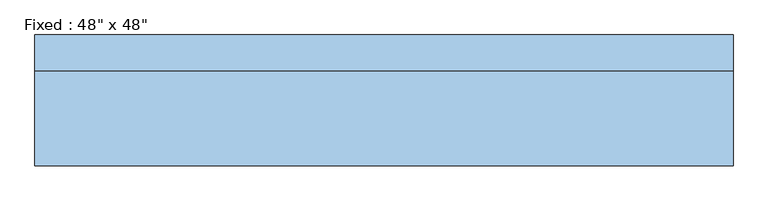
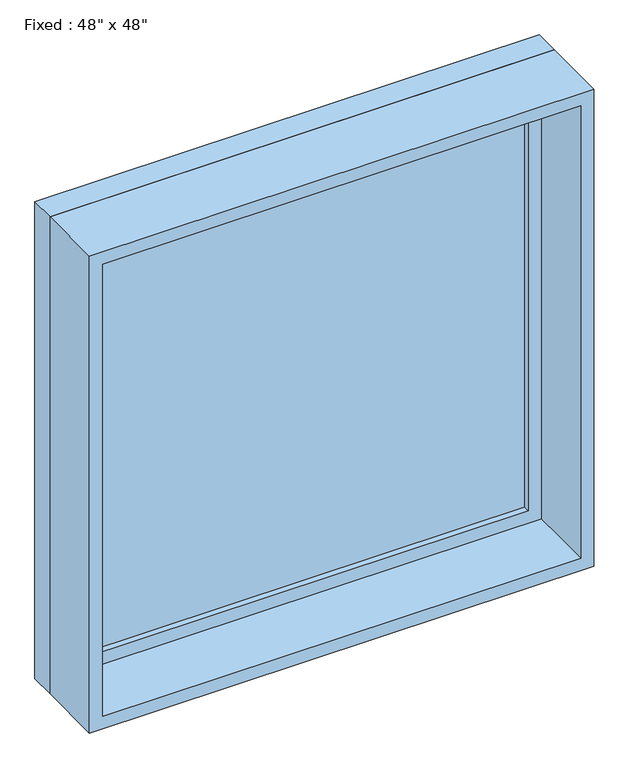
"""IFC4 building model written with IfcOpenShell, lengths in millimetres: window geometry."""

from ifc_helpers import new_model, si_unit, frame, origin, place, context, project, spatial, polyline, outline, extrude, source, transform, mapped, element, save


def window_76f305d9(model_context):
    return source(origin(), model_context, "Body", "SweptSolid", [
        extrude(outline(polyline([(508.0, 66.675), (-584.2, 66.675), (-584.2, 79.375), (508.0, 79.375), (508.0, 66.675)])), frame((0.0, 0.0, 977.9), z_axis=(0.0, 0.0, 1.0), x_axis=(1.0, 0.0, 0.0)), (0.0, 0.0, 1.0), 1092.2),
        extrude(outline(polyline([(2114.55, -628.65), (933.45, -628.65), (933.45, 552.45), (2114.55, 552.45), (2114.55, -628.65)]), holes=[polyline([(2070.1, -584.2), (2070.1, 508.0), (977.9, 508.0), (977.9, -584.2), (2070.1, -584.2)])]), frame((0.0, 50.8, 0.0), z_axis=(0.0, 1.0, 0.0), x_axis=(0.0, 0.0, 1.0)), (0.0, 0.0, 1.0), 44.45),
        extrude(outline(polyline([(2133.6, -647.7), (914.4, -647.7), (914.4, 571.5), (2133.6, 571.5), (2133.6, -647.7)]), holes=[polyline([(2101.85, -615.95), (2101.85, 539.75), (946.15, 539.75), (946.15, -615.95), (2101.85, -615.95)])]), frame((0.0, -114.3, 0.0), z_axis=(0.0, 1.0, 0.0), x_axis=(0.0, 0.0, 1.0)), (0.0, 0.0, 1.0), 165.1),
        extrude(outline(polyline([(2133.6, 571.5), (2133.6, -647.7), (914.4, -647.7), (914.4, 571.5), (2133.6, 571.5)]), holes=[polyline([(2114.55, 552.45), (933.45, 552.45), (933.45, -628.65), (2114.55, -628.65), (2114.55, 552.45)])]), frame((0.0, 50.8, 0.0), z_axis=(0.0, 1.0, 0.0), x_axis=(0.0, 0.0, 1.0)), (0.0, 0.0, 1.0), 63.5),
    ])


if __name__ == "__main__":
    model = new_model("IFC4")
    model_context = context("Model", 3, world=origin())
    ifc_project = project(units=[si_unit("LENGTHUNIT", "METRE", prefix="MILLI")], contexts=[model_context])
    site = spatial("IfcSite", under=ifc_project)
    building = spatial("IfcBuilding", under=site)
    placement = place(None, origin())
    window_shape = window_76f305d9(model_context)
    element("IfcWindow", 1, ObjectType="Fixed : 48\" x 48\"", at=placement, inside=building, context=model_context, shape_type="MappedRepresentation", body=[
        mapped(window_shape, transform((0.0, 0.0, 0.0), x_axis=(1.0, 0.0, 0.0), y_axis=(0.0, 1.0, 0.0), z_axis=(0.0, 0.0, 1.0))),
    ])
    save(model, "model.ifc")

# Revit data of these elements
# Type "Fixed : 48\" x 48\""
#   Type Mark = "2"
#   Assembly Code = "B2020100"
#   Height = 4' - 0"
#   Default Sill Height = 3' - 0"
#   Width = 4' - 0"
#   Window Inset = 0' - 0 3/4"
#   Glass Pane Material = Glass
#   Sash Material = Sash
#   Wall Closure = (empty or 0)
# Element 1 (IfcWindow, "Fixed : 48\" x 48\"")
#   Materials on its faces: "Sash", "Glass"
# Materials
#   "Glass": class "Glass", colour RGB 218 227 224, transparency 0.85, Description = "Soda Lime Glass", Cost = 0
#   "Sash": class "Wood", colour RGB 136 99 55, transparency 0
